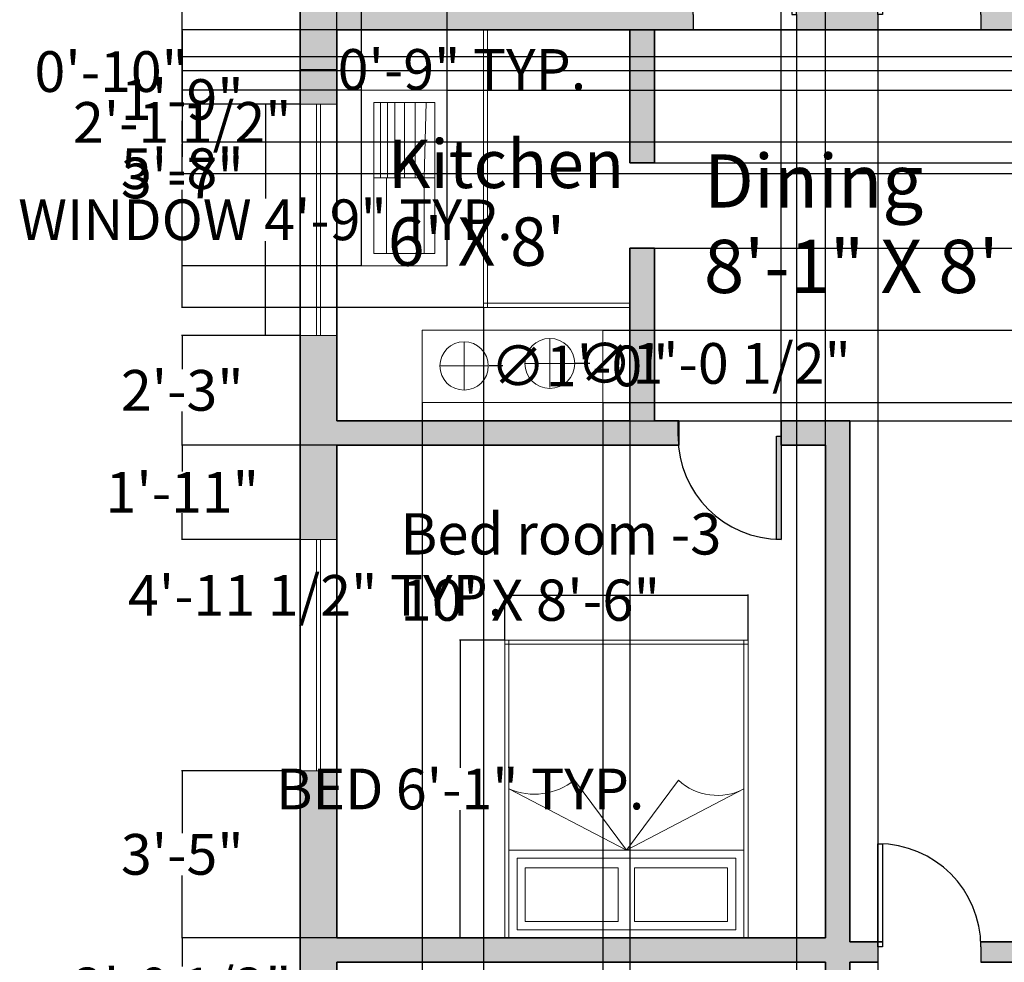
# Model space of a CAD drawing. Units: inches. Extents: x 46 to 946, y 121 to 740.
# Tile 2 of 4: x 46 to 287, y 299 to 531. Entities that reach past the tile are written whole.
import ezdxf

# ---------------------------------------------------------------- set-up
doc = ezdxf.new("R2010")
doc.units = ezdxf.units.IN
doc.header["$MEASUREMENT"] = 0
for name, color, linetype, lineweight in [('A-ANNO-DIMS', 2, 'Continuous', 18), ('A-AREA-IDEN', 7, 'Continuous', 25), ('A-DOOR', 3, 'Continuous', 25), ('A-EQPM', 9, 'Continuous', 18), ('A-FLOR-CASE', 8, 'Continuous', 18), ('A-FLOR-FIXT', 9, 'Continuous', 18), ('A-FURN', 8, 'Continuous', 18), ('A-GLAZ', 4, 'Continuous', 18), ('A-WALL', 7, 'Continuous', 35), ('A-WALL-PATT', 8, 'Continuous', 13)]:
    doc.layers.add(name, color=color, linetype=linetype, lineweight=lineweight)
doc.styles.get("Standard").update_dxf_attribs({"font": 'arial.ttf'})
doc.dimstyles.get("Standard").update_dxf_attribs({"dimtxt": 10, "dimasz": 0.18, "dimexe": 0.18, "dimexo": 0.0625, "dimgap": 0.09, "dimtad": 0, "dimtih": 1, "dimtoh": 1, "dimdec": 0, "dimzin": 0, "dimdsep": 46, "dimlunit": 3, "dimtxsty": 'Standard', "dimcen": 0.09, "dimadec": 0, "dimazin": 0, "dimtfac": 1, "dimtdec": 0, "dimtofl": 0, "dimtmove": 0, "dimatfit": 3, "dimfxl": 1, "dimtolj": 1, "dimtzin": 0, "dimarcsym": 0})

# ---------------------------------------------------------------- blocks, each defined once
blk = doc.blocks.new('*U3')
for p, q in [((0, 0), (0, -6)), ((40, 0), (40, -6))]:
    blk.add_line(p, q)
blk.add_lwpolyline([(0, 0), (0, 40), (1.75, 40), (1.75, 0)], close=True)
blk.add_arc((0, 0), 40, 0, 90)
blk = doc.blocks.new('WIN-56_82IN')
for p, q in [((9, 56.82), (0, 56.82)), ((0, 0), (0, 56.82)), ((4, 56.82), (4, 0)), ((5, 56.82), (5, 0)), ((9, 56.82), (9, 0)), ((9, 0), (0, 0))]:
    blk.add_line(p, q)
blk = doc.blocks.new('BED-DOUBLE')
for p, q in [((0, 73.15), (0, 0)), ((1, 73.15), (1, 0)), ((58.72, 0), (58.72, 73.15)), ((59.72, 0), (59.72, 73.15)), ((29.86, 51.59), (1, 36.57)), ((29.86, 51.59), (17.08, 34.42)), ((29.86, 51.59), (58.72, 36.57)), ((29.86, 51.59), (42.63, 34.42)), ((0, 1), (59.72, 1)), ((0, 0), (59.72, 0))]:
    blk.add_line(p, q)
for points in [[(1, 73.15), (58.72, 73.15), (58.72, 51.59), (1, 51.59)], [(3, 71.15), (56.72, 71.15), (56.72, 53.59), (3, 53.59)], [(5, 69.15), (27.85, 69.15), (27.85, 55.92), (5, 55.92)], [(54.72, 69.15), (31.87, 69.15), (31.87, 55.92), (54.72, 55.92)]]:
    blk.add_lwpolyline(points, close=True)
for centre, radius, start, end in [((7.51, 24.06), 14.1, 47.2425, 117.4957), ((52.47, 22.1), 15.76, 66.6553, 128.6065)]:
    blk.add_arc(centre, radius, start, end)
blk = doc.blocks.new('*D18')
at = {"layer": 'A-ANNO-DIMS', "color": 0, "lineweight": -2, "transparency": 16777216}
for p, q in [((114.41, 510.24), (105.77, 510.24)), ((105.95, 510.06), (105.95, 487.09)), ((105.95, 453.6), (105.95, 476.56)), ((114.41, 453.42), (105.77, 453.42))]:
    blk.add_line(p, q, dxfattribs=at)
at = {"layer": 'A-ANNO-DIMS', "color": 0, "transparency": 16777216}
for points in [[(105.92, 510.06), (105.98, 510.06), (105.95, 510.24)], [(105.92, 453.6), (105.98, 453.6), (105.95, 453.42)]]:
    blk.add_solid(points, dxfattribs=at)
at = {"layer": 'Defpoints', "color": 0, "transparency": 16777216}
for p in [(105.95, 510.24), (114.48, 510.24), (114.48, 453.42)]:
    blk.add_point(p, dxfattribs=at)
at = {"layer": 'A-ANNO-DIMS', "color": 0, "transparency": 16777216, "insert": (105.95, 481.83), "char_height": 10, "attachment_point": 5}
blk.add_mtext('\\A1;WINDOW 4\'-9" TYP.', dxfattribs=at)
blk = doc.blocks.new('*D19')
at = {"layer": 'A-ANNO-DIMS', "color": 0, "lineweight": -2, "transparency": 16777216}
for p, q in [((114.48, 510.3), (114.48, 518.94)), ((114.66, 518.76), (123.3, 518.76)), ((123.48, 510.3), (123.48, 518.94)), ((123.48, 518.76), (123.66, 518.76))]:
    blk.add_line(p, q, dxfattribs=at)
at = {"layer": 'A-ANNO-DIMS', "color": 0, "transparency": 16777216}
for points in [[(114.66, 518.79), (114.66, 518.73), (114.48, 518.76)], [(123.3, 518.79), (123.3, 518.73), (123.48, 518.76)]]:
    blk.add_solid(points, dxfattribs=at)
at = {"layer": 'Defpoints', "color": 0, "transparency": 16777216}
for p in [(123.48, 518.76), (114.48, 510.24), (123.48, 510.24)]:
    blk.add_point(p, dxfattribs=at)
at = {"layer": 'A-ANNO-DIMS', "color": 0, "transparency": 16777216, "insert": (154.22, 518.76), "char_height": 10, "attachment_point": 5}
blk.add_mtext('\\A1;0\'-9" TYP.', dxfattribs=at)
blk = doc.blocks.new('*D22')
at = {"layer": 'A-ANNO-DIMS', "color": 0, "lineweight": -2, "transparency": 16777216}
for p, q in [((164.7, 378.61), (153.61, 378.61)), ((153.79, 378.43), (153.79, 347.23)), ((153.79, 305.64), (153.79, 336.84)), ((164.7, 305.46), (153.61, 305.46))]:
    blk.add_line(p, q, dxfattribs=at)
at = {"layer": 'A-ANNO-DIMS', "color": 0, "transparency": 16777216}
for points in [[(153.76, 378.43), (153.82, 378.43), (153.79, 378.61)], [(153.76, 305.64), (153.82, 305.64), (153.79, 305.46)]]:
    blk.add_solid(points, dxfattribs=at)
at = {"layer": 'Defpoints', "color": 0, "transparency": 16777216}
for p in [(164.76, 378.61), (153.79, 305.46), (164.76, 305.46)]:
    blk.add_point(p, dxfattribs=at)
at = {"layer": 'A-ANNO-DIMS', "color": 0, "transparency": 16777216, "insert": (153.79, 342.03), "char_height": 10, "attachment_point": 5}
blk.add_mtext('\\A1;BED 6\'-1" TYP.', dxfattribs=at)
blk = doc.blocks.new('*D23')
at = {"layer": 'A-ANNO-DIMS', "color": 0, "lineweight": -2, "transparency": 16777216}
for p, q in [((164.76, 389.58), (164.58, 389.58)), ((164.76, 378.67), (164.76, 389.76)), ((224.3, 389.58), (164.94, 389.58)), ((224.48, 378.67), (224.48, 389.76))]:
    blk.add_line(p, q, dxfattribs=at)
at = {"layer": 'A-ANNO-DIMS', "color": 0, "transparency": 16777216}
for points in [[(164.94, 389.61), (164.94, 389.55), (164.76, 389.58)], [(224.3, 389.61), (224.3, 389.55), (224.48, 389.58)]]:
    blk.add_solid(points, dxfattribs=at)
at = {"layer": 'Defpoints', "color": 0, "transparency": 16777216}
for p in [(164.76, 389.58), (164.76, 378.61), (224.48, 378.61)]:
    blk.add_point(p, dxfattribs=at)
at = {"layer": 'A-ANNO-DIMS', "color": 0, "transparency": 16777216, "insert": (118.28, 389.58), "char_height": 10, "attachment_point": 5}
blk.add_mtext('\\A1;4\'-11 1/2" TYP.', dxfattribs=at)
blk = doc.blocks.new('*D32')
at = {"layer": 'A-ANNO-DIMS', "color": 0, "lineweight": -2, "transparency": 16777216}
for p, q in [((123.41, 305.46), (85.35, 305.46)), ((85.53, 305.28), (85.53, 298.41)), ((85.53, 281.01), (85.53, 287.89)), ((114.41, 280.83), (85.35, 280.83))]:
    blk.add_line(p, q, dxfattribs=at)
at = {"layer": 'A-ANNO-DIMS', "color": 0, "transparency": 16777216}
for points in [[(85.5, 305.28), (85.56, 305.28), (85.53, 305.46)], [(85.5, 281.01), (85.56, 281.01), (85.53, 280.83)]]:
    blk.add_solid(points, dxfattribs=at)
at = {"layer": 'Defpoints', "color": 0, "transparency": 16777216}
for p in [(85.53, 305.46), (123.48, 305.46), (114.48, 280.83)]:
    blk.add_point(p, dxfattribs=at)
at = {"layer": 'A-ANNO-DIMS', "color": 0, "transparency": 16777216, "insert": (85.53, 293.15), "char_height": 10, "attachment_point": 5}
blk.add_mtext('\\A1;2\'-0 1/2"', dxfattribs=at)
blk = doc.blocks.new('*D33')
at = {"layer": 'A-ANNO-DIMS', "color": 0, "lineweight": -2, "transparency": 16777216}
for p, q in [((114.41, 346.49), (85.35, 346.49)), ((85.53, 346.31), (85.53, 331.17)), ((85.53, 305.64), (85.53, 320.78)), ((123.41, 305.46), (85.35, 305.46))]:
    blk.add_line(p, q, dxfattribs=at)
at = {"layer": 'A-ANNO-DIMS', "color": 0, "transparency": 16777216}
for points in [[(85.5, 346.31), (85.56, 346.31), (85.53, 346.49)], [(85.5, 305.64), (85.56, 305.64), (85.53, 305.46)]]:
    blk.add_solid(points, dxfattribs=at)
at = {"layer": 'Defpoints', "color": 0, "transparency": 16777216}
for p in [(85.53, 346.49), (114.48, 346.49), (123.48, 305.46)]:
    blk.add_point(p, dxfattribs=at)
at = {"layer": 'A-ANNO-DIMS', "color": 0, "transparency": 16777216, "insert": (85.53, 325.98), "char_height": 10, "attachment_point": 5}
blk.add_mtext('\\A1;3\'-5"', dxfattribs=at)
blk = doc.blocks.new('*D34')
at = {"layer": 'A-ANNO-DIMS', "color": 0, "lineweight": -2, "transparency": 16777216}
for p, q in [((123.41, 426.46), (85.35, 426.46)), ((85.53, 426.28), (85.53, 420)), ((85.53, 403.49), (85.53, 409.78)), ((114.41, 403.31), (85.35, 403.31))]:
    blk.add_line(p, q, dxfattribs=at)
at = {"layer": 'A-ANNO-DIMS', "color": 0, "transparency": 16777216}
for points in [[(85.5, 426.28), (85.56, 426.28), (85.53, 426.46)], [(85.5, 403.49), (85.56, 403.49), (85.53, 403.31)]]:
    blk.add_solid(points, dxfattribs=at)
at = {"layer": 'Defpoints', "color": 0, "transparency": 16777216}
for p in [(85.53, 426.46), (123.48, 426.46), (114.48, 403.31)]:
    blk.add_point(p, dxfattribs=at)
at = {"layer": 'A-ANNO-DIMS', "color": 0, "transparency": 16777216, "insert": (85.53, 414.89), "char_height": 10, "attachment_point": 5}
blk.add_mtext('\\A1;1\'-11"', dxfattribs=at)
blk = doc.blocks.new('*D35')
at = {"layer": 'A-ANNO-DIMS', "color": 0, "lineweight": -2, "transparency": 16777216}
for p, q in [((114.41, 453.42), (85.35, 453.42)), ((85.53, 453.24), (85.53, 445.14)), ((85.53, 426.64), (85.53, 434.74)), ((123.41, 426.46), (85.35, 426.46))]:
    blk.add_line(p, q, dxfattribs=at)
at = {"layer": 'A-ANNO-DIMS', "color": 0, "transparency": 16777216}
for points in [[(85.5, 453.24), (85.56, 453.24), (85.53, 453.42)], [(85.5, 426.64), (85.56, 426.64), (85.53, 426.46)]]:
    blk.add_solid(points, dxfattribs=at)
at = {"layer": 'Defpoints', "color": 0, "transparency": 16777216}
for p in [(85.53, 453.42), (114.48, 453.42), (123.48, 426.46)]:
    blk.add_point(p, dxfattribs=at)
at = {"layer": 'A-ANNO-DIMS', "color": 0, "transparency": 16777216, "insert": (85.53, 439.94), "char_height": 10, "attachment_point": 5}
blk.add_mtext('\\A1;2\'-3"', dxfattribs=at)
blk = doc.blocks.new('*D36')
at = {"layer": 'A-ANNO-DIMS', "color": 0, "lineweight": -2, "transparency": 16777216}
for p, q in [((114.41, 573.18), (85.35, 573.18)), ((85.53, 573), (85.53, 546.91)), ((85.53, 510.42), (85.53, 536.51)), ((114.41, 510.24), (85.35, 510.24))]:
    blk.add_line(p, q, dxfattribs=at)
at = {"layer": 'A-ANNO-DIMS', "color": 0, "transparency": 16777216}
for points in [[(85.5, 573), (85.56, 573), (85.53, 573.18)], [(85.5, 510.42), (85.56, 510.42), (85.53, 510.24)]]:
    blk.add_solid(points, dxfattribs=at)
at = {"layer": 'Defpoints', "color": 0, "transparency": 16777216}
for p in [(85.53, 573.18), (114.48, 573.18), (114.48, 510.24)]:
    blk.add_point(p, dxfattribs=at)
at = {"layer": 'A-ANNO-DIMS', "color": 0, "transparency": 16777216, "insert": (85.53, 541.71), "char_height": 10, "attachment_point": 5}
blk.add_mtext('\\A1;5\'-3"', dxfattribs=at)
blk = doc.blocks.new('*D45')
at = {"layer": 'A-ANNO-DIMS', "color": 0, "lineweight": -2, "transparency": 16777216}
for p, q in [((129.58, 470.61), (129.58, 722.59)), ((129.76, 722.41), (150.42, 722.41)), ((150.6, 470.61), (150.6, 722.59)), ((150.6, 722.41), (150.78, 722.41))]:
    blk.add_line(p, q, dxfattribs=at)
at = {"layer": 'A-ANNO-DIMS', "color": 0, "transparency": 16777216}
for points in [[(129.76, 722.44), (129.76, 722.38), (129.58, 722.41)], [(150.42, 722.44), (150.42, 722.38), (150.6, 722.41)]]:
    blk.add_solid(points, dxfattribs=at)
at = {"layer": 'Defpoints', "color": 0, "transparency": 16777216}
for p in [(150.6, 722.41), (129.58, 470.54), (150.6, 470.54)]:
    blk.add_point(p, dxfattribs=at)
at = {"layer": 'A-ANNO-DIMS', "color": 0, "transparency": 16777216, "insert": (163.69, 722.41), "char_height": 10, "attachment_point": 5}
blk.add_mtext('\\A1;1\'-9"', dxfattribs=at)
blk = doc.blocks.new('*D46')
at = {"layer": 'A-ANNO-DIMS', "color": 0, "lineweight": -2, "transparency": 16777216}
for p, q in [((129.52, 513.68), (85.35, 513.68)), ((85.53, 513.5), (85.53, 497.31)), ((85.53, 470.72), (85.53, 486.91)), ((129.52, 470.54), (85.35, 470.54))]:
    blk.add_line(p, q, dxfattribs=at)
at = {"layer": 'A-ANNO-DIMS', "color": 0, "transparency": 16777216}
for points in [[(85.5, 513.5), (85.56, 513.5), (85.53, 513.68)], [(85.5, 470.72), (85.56, 470.72), (85.53, 470.54)]]:
    blk.add_solid(points, dxfattribs=at)
at = {"layer": 'Defpoints', "color": 0, "transparency": 16777216}
for p in [(85.53, 513.68), (129.58, 513.68), (129.58, 470.54)]:
    blk.add_point(p, dxfattribs=at)
at = {"layer": 'A-ANNO-DIMS', "color": 0, "transparency": 16777216, "insert": (85.53, 492.11), "char_height": 10, "attachment_point": 5}
blk.add_mtext('\\A1;3\'-7"', dxfattribs=at)
blk = doc.blocks.new('*D47')
at = {"layer": 'A-ANNO-DIMS', "color": 0, "lineweight": -2, "transparency": 16777216}
for p, q in [((144.44, 436.91), (144.44, 135.33)), ((188.83, 436.91), (188.83, 135.33)), ((144.62, 135.51), (188.65, 135.51)), ((188.83, 135.51), (189.01, 135.51))]:
    blk.add_line(p, q, dxfattribs=at)
at = {"layer": 'A-ANNO-DIMS', "color": 0, "transparency": 16777216}
for points in [[(144.62, 135.54), (144.62, 135.48), (144.44, 135.51)], [(188.65, 135.54), (188.65, 135.48), (188.83, 135.51)]]:
    blk.add_solid(points, dxfattribs=at)
at = {"layer": 'Defpoints', "color": 0, "transparency": 16777216}
for p in [(144.44, 436.97), (188.83, 436.97), (188.83, 135.51)]:
    blk.add_point(p, dxfattribs=at)
at = {"layer": 'A-ANNO-DIMS', "color": 0, "transparency": 16777216, "insert": (214.03, 135.51), "char_height": 10, "attachment_point": 5}
blk.add_mtext('\\A1;3\'-8 1/2"', dxfattribs=at)
blk = doc.blocks.new('*D48')
at = {"layer": 'A-ANNO-DIMS', "color": 0, "lineweight": -2, "transparency": 16777216}
for p, q in [((188.89, 454.75), (482.61, 454.75)), ((482.43, 454.57), (482.43, 451.05)), ((482.43, 437.15), (482.43, 440.66)), ((188.89, 436.97), (482.61, 436.97))]:
    blk.add_line(p, q, dxfattribs=at)
at = {"layer": 'A-ANNO-DIMS', "color": 0, "transparency": 16777216}
for points in [[(482.4, 454.57), (482.46, 454.57), (482.43, 454.75)], [(482.4, 437.15), (482.46, 437.15), (482.43, 436.97)]]:
    blk.add_solid(points, dxfattribs=at)
at = {"layer": 'Defpoints', "color": 0, "transparency": 16777216}
for p in [(188.83, 454.75), (482.43, 454.75), (188.83, 436.97)]:
    blk.add_point(p, dxfattribs=at)
at = {"layer": 'A-ANNO-DIMS', "color": 0, "transparency": 16777216, "insert": (482.43, 445.86), "char_height": 10, "attachment_point": 5}
blk.add_mtext('\\A1;1\'-6"', dxfattribs=at)
blk = doc.blocks.new('*D49')
at = {"layer": 'A-ANNO-DIMS', "color": 0, "lineweight": -2, "transparency": 16777216}
for p, q in [((159.48, 460.26), (159.48, 135.33)), ((195.48, 460.26), (195.48, 135.33)), ((159.66, 135.51), (164.1, 135.51)), ((195.3, 135.51), (190.85, 135.51))]:
    blk.add_line(p, q, dxfattribs=at)
at = {"layer": 'A-ANNO-DIMS', "color": 0, "transparency": 16777216}
for points in [[(159.66, 135.54), (159.66, 135.48), (159.48, 135.51)], [(195.3, 135.54), (195.3, 135.48), (195.48, 135.51)]]:
    blk.add_solid(points, dxfattribs=at)
at = {"layer": 'Defpoints', "color": 0, "transparency": 16777216}
for p in [(159.48, 460.32), (195.48, 460.32), (195.48, 135.51)]:
    blk.add_point(p, dxfattribs=at)
at = {"layer": 'A-ANNO-DIMS', "color": 0, "transparency": 16777216, "insert": (177.48, 135.51), "char_height": 10, "attachment_point": 5}
blk.add_mtext('\\A1;3\'-0"', dxfattribs=at)
blk = doc.blocks.new('*D50')
at = {"layer": 'A-ANNO-DIMS', "color": 0, "lineweight": -2, "transparency": 16777216}
for p, q in [((195.54, 495.84), (482.61, 495.84)), ((482.43, 495.66), (482.43, 490.57)), ((482.43, 475.08), (482.43, 480.18)), ((195.54, 474.9), (482.61, 474.9))]:
    blk.add_line(p, q, dxfattribs=at)
at = {"layer": 'A-ANNO-DIMS', "color": 0, "transparency": 16777216}
for points in [[(482.4, 495.66), (482.46, 495.66), (482.43, 495.84)], [(482.4, 475.08), (482.46, 475.08), (482.43, 474.9)]]:
    blk.add_solid(points, dxfattribs=at)
at = {"layer": 'Defpoints', "color": 0, "transparency": 16777216}
for p in [(195.48, 495.84), (482.43, 495.84), (195.48, 474.9)]:
    blk.add_point(p, dxfattribs=at)
at = {"layer": 'A-ANNO-DIMS', "color": 0, "transparency": 16777216, "insert": (482.43, 485.37), "char_height": 10, "attachment_point": 5}
blk.add_mtext('\\A1;1\'-9"', dxfattribs=at)
blk = doc.blocks.new('*D60')
at = {"layer": 'A-ANNO-DIMS', "color": 0, "lineweight": -2, "transparency": 16777216}
for p, q in [((385.41, 521.87), (85.35, 521.87)), ((85.53, 521.69), (85.53, 516.57)), ((85.53, 501.05), (85.53, 506.18)), ((385.41, 500.87), (85.35, 500.87))]:
    blk.add_line(p, q, dxfattribs=at)
at = {"layer": 'A-ANNO-DIMS', "color": 0, "transparency": 16777216}
for points in [[(85.5, 521.69), (85.56, 521.69), (85.53, 521.87)], [(85.5, 501.05), (85.56, 501.05), (85.53, 500.87)]]:
    blk.add_solid(points, dxfattribs=at)
at = {"layer": 'Defpoints', "color": 0, "transparency": 16777216}
for p in [(85.53, 521.87), (385.48, 521.87), (385.48, 500.87)]:
    blk.add_point(p, dxfattribs=at)
at = {"layer": 'A-ANNO-DIMS', "color": 0, "transparency": 16777216, "insert": (85.53, 511.37), "char_height": 10, "attachment_point": 5}
blk.add_mtext('\\A1;1\'-9"', dxfattribs=at)
blk = doc.blocks.new('*D61')
at = {"layer": 'A-ANNO-DIMS', "color": 0, "lineweight": -2, "transparency": 16777216}
for p, q in [((304.41, 528.46), (85.35, 528.46)), ((85.53, 528.28), (85.53, 518.59)), ((298.41, 518.41), (85.35, 518.41)), ((85.53, 518.23), (85.35, 518.23)), ((85.53, 518.41), (85.53, 518.23))]:
    blk.add_line(p, q, dxfattribs=at)
at = {"layer": 'A-ANNO-DIMS', "color": 0, "transparency": 16777216}
for points in [[(85.5, 528.28), (85.56, 528.28), (85.53, 528.46)], [(85.5, 518.59), (85.56, 518.59), (85.53, 518.41)]]:
    blk.add_solid(points, dxfattribs=at)
at = {"layer": 'Defpoints', "color": 0, "transparency": 16777216}
for p in [(304.48, 528.46), (85.53, 518.41), (298.48, 518.41)]:
    blk.add_point(p, dxfattribs=at)
at = {"layer": 'A-ANNO-DIMS', "color": 0, "transparency": 16777216, "insert": (68.08, 518.23), "char_height": 10, "attachment_point": 5}
blk.add_mtext('\\A1;0\'-10"', dxfattribs=at)
blk = doc.blocks.new('*D62')
at = {"layer": 'A-ANNO-DIMS', "color": 0, "lineweight": -2, "transparency": 16777216}
for p, q in [((298.41, 518.41), (85.35, 518.41)), ((85.53, 518.23), (85.53, 511.01)), ((85.53, 493.27), (85.53, 500.49)), ((298.41, 493.09), (85.35, 493.09))]:
    blk.add_line(p, q, dxfattribs=at)
at = {"layer": 'A-ANNO-DIMS', "color": 0, "transparency": 16777216}
for points in [[(85.5, 518.23), (85.56, 518.23), (85.53, 518.41)], [(85.5, 493.27), (85.56, 493.27), (85.53, 493.09)]]:
    blk.add_solid(points, dxfattribs=at)
at = {"layer": 'Defpoints', "color": 0, "transparency": 16777216}
for p in [(298.48, 518.41), (85.53, 493.09), (298.48, 493.09)]:
    blk.add_point(p, dxfattribs=at)
at = {"layer": 'A-ANNO-DIMS', "color": 0, "transparency": 16777216, "insert": (85.53, 505.75), "char_height": 10, "attachment_point": 5}
blk.add_mtext('\\A1;2\'-1 1/2"', dxfattribs=at)
blk = doc.blocks.new('*D63')
at = {"layer": 'A-ANNO-DIMS', "color": 0, "lineweight": -2, "transparency": 16777216}
for p, q in [((195.54, 528.46), (482.61, 528.46)), ((482.43, 528.28), (482.43, 517.41)), ((482.43, 496.02), (482.43, 506.89)), ((195.54, 495.84), (482.61, 495.84))]:
    blk.add_line(p, q, dxfattribs=at)
at = {"layer": 'A-ANNO-DIMS', "color": 0, "transparency": 16777216}
for points in [[(482.4, 528.28), (482.46, 528.28), (482.43, 528.46)], [(482.4, 496.02), (482.46, 496.02), (482.43, 495.84)]]:
    blk.add_solid(points, dxfattribs=at)
at = {"layer": 'Defpoints', "color": 0, "transparency": 16777216}
for p in [(195.48, 528.46), (195.48, 495.84), (482.43, 495.84)]:
    blk.add_point(p, dxfattribs=at)
at = {"layer": 'A-ANNO-DIMS', "color": 0, "transparency": 16777216, "insert": (482.43, 512.15), "char_height": 10, "attachment_point": 5}
blk.add_mtext('\\A1;2\'-8 1/2"', dxfattribs=at)
blk = doc.blocks.new('*D64')
at = {"layer": 'A-ANNO-DIMS', "color": 0, "lineweight": -2, "transparency": 16777216}
for p, q in [((188.83, 436.91), (188.83, 135.33)), ((195.48, 432.4), (195.48, 135.33)), ((188.83, 135.51), (188.65, 135.51)), ((195.3, 135.51), (189.01, 135.51))]:
    blk.add_line(p, q, dxfattribs=at)
at = {"layer": 'A-ANNO-DIMS', "color": 0, "transparency": 16777216}
for points in [[(189.01, 135.54), (189.01, 135.48), (188.83, 135.51)], [(195.3, 135.54), (195.3, 135.48), (195.48, 135.51)]]:
    blk.add_solid(points, dxfattribs=at)
at = {"layer": 'Defpoints', "color": 0, "transparency": 16777216}
for p in [(188.83, 436.97), (195.48, 432.46), (188.83, 135.51)]:
    blk.add_point(p, dxfattribs=at)
at = {"layer": 'A-ANNO-DIMS', "color": 0, "transparency": 16777216, "insert": (163.61, 135.51), "char_height": 10, "attachment_point": 5}
blk.add_mtext('\\A1;0\'-6 1/2"', dxfattribs=at)
blk = doc.blocks.new('*D65')
at = {"layer": 'A-ANNO-DIMS', "color": 0, "lineweight": -2, "transparency": 16777216}
for p, q in [((232.61, 426.52), (232.61, 722.59)), ((232.79, 722.41), (243.3, 722.41)), ((243.48, 426.52), (243.48, 722.59)), ((243.48, 722.41), (243.66, 722.41))]:
    blk.add_line(p, q, dxfattribs=at)
at = {"layer": 'A-ANNO-DIMS', "color": 0, "transparency": 16777216}
for points in [[(232.79, 722.44), (232.79, 722.38), (232.61, 722.41)], [(243.3, 722.44), (243.3, 722.38), (243.48, 722.41)]]:
    blk.add_solid(points, dxfattribs=at)
at = {"layer": 'Defpoints', "color": 0, "transparency": 16777216}
for p in [(243.48, 722.41), (232.61, 426.46), (243.48, 426.46)]:
    blk.add_point(p, dxfattribs=at)
at = {"layer": 'A-ANNO-DIMS', "color": 0, "transparency": 16777216, "insert": (260.92, 722.41), "char_height": 10, "attachment_point": 5}
blk.add_mtext('\\A1;0\'-11"', dxfattribs=at)
blk = doc.blocks.new('*D66')
at = {"layer": 'A-ANNO-DIMS', "color": 0, "lineweight": -2, "transparency": 16777216}
for p, q in [((123.48, 528.52), (123.48, 722.59)), ((123.66, 722.41), (129.4, 722.41)), ((129.58, 513.74), (129.58, 722.59)), ((129.58, 722.41), (129.76, 722.41))]:
    blk.add_line(p, q, dxfattribs=at)
at = {"layer": 'A-ANNO-DIMS', "color": 0, "transparency": 16777216}
for points in [[(123.66, 722.44), (123.66, 722.38), (123.48, 722.41)], [(129.4, 722.44), (129.4, 722.38), (129.58, 722.41)]]:
    blk.add_solid(points, dxfattribs=at)
at = {"layer": 'Defpoints', "color": 0, "transparency": 16777216}
for p in [(129.58, 722.41), (123.48, 528.46), (129.58, 513.68)]:
    blk.add_point(p, dxfattribs=at)
at = {"layer": 'A-ANNO-DIMS', "color": 0, "transparency": 16777216, "insert": (143.14, 722.41), "char_height": 10, "attachment_point": 5}
blk.add_mtext('\\A1;0\'-6"', dxfattribs=at)
blk = doc.blocks.new('*D67')
at = {"layer": 'A-ANNO-DIMS', "color": 0, "lineweight": -2, "transparency": 16777216}
for p, q in [((159.54, 528.46), (482.61, 528.46)), ((482.43, 528.28), (482.43, 526.27)), ((482.43, 513.86), (482.43, 515.87)), ((150.66, 513.68), (482.61, 513.68))]:
    blk.add_line(p, q, dxfattribs=at)
at = {"layer": 'A-ANNO-DIMS', "color": 0, "transparency": 16777216}
for points in [[(482.4, 528.28), (482.46, 528.28), (482.43, 528.46)], [(482.4, 513.86), (482.46, 513.86), (482.43, 513.68)]]:
    blk.add_solid(points, dxfattribs=at)
at = {"layer": 'Defpoints', "color": 0, "transparency": 16777216}
for p in [(159.48, 528.46), (482.43, 528.46), (150.6, 513.68)]:
    blk.add_point(p, dxfattribs=at)
at = {"layer": 'A-ANNO-DIMS', "color": 0, "transparency": 16777216, "insert": (482.43, 521.07), "char_height": 10, "attachment_point": 5}
blk.add_mtext('\\A1;1\'-3"', dxfattribs=at)
blk = doc.blocks.new('*D68')
at = {"layer": 'A-ANNO-DIMS', "color": 0, "lineweight": -2, "transparency": 16777216}
for p, q in [((159.41, 528.46), (85.35, 528.46)), ((85.53, 528.28), (85.53, 499.59)), ((85.53, 460.5), (85.53, 489.2)), ((159.41, 460.32), (85.35, 460.32))]:
    blk.add_line(p, q, dxfattribs=at)
at = {"layer": 'A-ANNO-DIMS', "color": 0, "transparency": 16777216}
for points in [[(85.5, 528.28), (85.56, 528.28), (85.53, 528.46)], [(85.5, 460.5), (85.56, 460.5), (85.53, 460.32)]]:
    blk.add_solid(points, dxfattribs=at)
at = {"layer": 'Defpoints', "color": 0, "transparency": 16777216}
for p in [(159.48, 528.46), (85.53, 460.32), (159.48, 460.32)]:
    blk.add_point(p, dxfattribs=at)
at = {"layer": 'A-ANNO-DIMS', "color": 0, "transparency": 16777216, "insert": (85.53, 494.39), "char_height": 10, "attachment_point": 5}
blk.add_mtext('\\A1;5\'-8"', dxfattribs=at)
blk = doc.blocks.new('*D69')
at = {"layer": 'A-ANNO-DIMS', "color": 0, "lineweight": -2, "transparency": 16777216}
for p, q in [((188.89, 436.97), (482.61, 436.97)), ((482.43, 436.79), (482.43, 432.64)), ((195.54, 432.46), (482.61, 432.46)), ((482.43, 432.28), (482.25, 432.28)), ((482.43, 432.46), (482.43, 432.28))]:
    blk.add_line(p, q, dxfattribs=at)
at = {"layer": 'A-ANNO-DIMS', "color": 0, "transparency": 16777216}
for points in [[(482.4, 436.79), (482.46, 436.79), (482.43, 436.97)], [(482.4, 432.64), (482.46, 432.64), (482.43, 432.46)]]:
    blk.add_solid(points, dxfattribs=at)
at = {"layer": 'Defpoints', "color": 0, "transparency": 16777216}
for p in [(188.83, 436.97), (195.48, 432.46), (482.43, 432.46)]:
    blk.add_point(p, dxfattribs=at)
at = {"layer": 'A-ANNO-DIMS', "color": 0, "transparency": 16777216, "insert": (457.21, 432.28), "char_height": 10, "attachment_point": 5}
blk.add_mtext('\\A1;0\'-4 1/2"', dxfattribs=at)
blk = doc.blocks.new('*D70')
at = {"layer": 'A-ANNO-DIMS', "color": 0, "lineweight": -2, "transparency": 16777216}
for p, q in [((236.36, 528.4), (236.36, 135.33)), ((256.37, 528.4), (256.37, 135.33)), ((236.54, 135.51), (256.19, 135.51)), ((256.37, 135.51), (256.55, 135.51))]:
    blk.add_line(p, q, dxfattribs=at)
at = {"layer": 'A-ANNO-DIMS', "color": 0, "transparency": 16777216}
for points in [[(236.54, 135.54), (236.54, 135.48), (236.36, 135.51)], [(256.19, 135.54), (256.19, 135.48), (256.37, 135.51)]]:
    blk.add_solid(points, dxfattribs=at)
at = {"layer": 'Defpoints', "color": 0, "transparency": 16777216}
for p in [(236.36, 528.46), (256.37, 528.46), (256.37, 135.51)]:
    blk.add_point(p, dxfattribs=at)
at = {"layer": 'A-ANNO-DIMS', "color": 0, "transparency": 16777216, "insert": (269.46, 135.51), "char_height": 10, "attachment_point": 5}
blk.add_mtext('\\A1;1\'-8"', dxfattribs=at)
blk = doc.blocks.new('*D71')
at = {"layer": 'A-ANNO-DIMS', "color": 0, "lineweight": -2, "transparency": 16777216}
for p, q in [((175.72, 446.56), (175.9, 446.56)), ((175.81, 446.47), (175.81, 446.65)), ((185.61, 446.56), (182.12, 446.56))]:
    blk.add_line(p, q, dxfattribs=at)
at = {"layer": 'A-ANNO-DIMS', "color": 0, "transparency": 16777216}
blk.add_solid([(182.12, 446.59), (182.12, 446.53), (181.94, 446.56)], dxfattribs=at)
at = {"layer": 'Defpoints', "color": 0, "transparency": 16777216}
for p in [(169.68, 446.56), (181.94, 446.56)]:
    blk.add_point(p, dxfattribs=at)
at = {"layer": 'A-ANNO-DIMS', "color": 0, "transparency": 16777216, "insert": (216.09, 446.56), "char_height": 10, "attachment_point": 5}
blk.add_mtext('\\A1;∅1\'-0 1/2"', dxfattribs=at)
blk = doc.blocks.new('*D72')
at = {"layer": 'A-ANNO-DIMS', "color": 0, "lineweight": -2, "transparency": 16777216}
for p, q in [((154.66, 445.94), (154.84, 445.94)), ((154.75, 445.85), (154.75, 446.03)), ((164.27, 445.94), (160.88, 445.94))]:
    blk.add_line(p, q, dxfattribs=at)
at = {"layer": 'A-ANNO-DIMS', "color": 0, "transparency": 16777216}
blk.add_solid([(160.88, 445.97), (160.88, 445.91), (160.7, 445.94)], dxfattribs=at)
at = {"layer": 'Defpoints', "color": 0, "transparency": 16777216}
for p in [(148.8, 445.94), (160.7, 445.94)]:
    blk.add_point(p, dxfattribs=at)
at = {"layer": 'A-ANNO-DIMS', "color": 0, "transparency": 16777216, "insert": (183.09, 445.94), "char_height": 10, "attachment_point": 5}
blk.add_mtext('\\A1;∅1\'-0"', dxfattribs=at)

msp = doc.modelspace()

# ---------------------------------------------------------------- hatches: boundary and pattern name
at = {"layer": 'A-WALL-PATT'}
h = msp.add_hatch(color=256, dxfattribs=at)
h.dxf.hatch_style = 1
h.paths.add_polyline_path([(256.37, 197.46), (249.48, 197.46), (249.48, 258.28), (245.68, 258.28, -0.021769), (243.48, 258.37), (243.48, 197.46), (221.61, 197.46), (221.61, 188.46), (243.48, 188.46), (256.37, 188.46), (256.37, 192.26)])
h.paths.add_polyline_path([(164.78, 197.46), (123.48, 197.46), (123.48, 224.01), (114.48, 224.01), (114.48, 188.46), (164.78, 188.46)])
h.paths.add_polyline_path([(402.48, 216.63), (393.48, 216.63), (393.48, 197.46), (327.48, 197.46), (281.15, 197.46, -0.051771), (281.69, 192.26), (281.69, 188.46), (402.48, 188.46)])
h.paths.add_polyline_path([(123.48, 346.49), (114.48, 346.49), (114.48, 280.83), (123.48, 280.83), (123.48, 299.46), (243.48, 299.46), (243.48, 283.6), (245.68, 283.6), (249.48, 283.6), (249.48, 299.46), (256.37, 299.46), (256.37, 303.26), (256.37, 304.46), (249.48, 304.46), (249.48, 432.46), (243.48, 432.46), (232.61, 432.46), (232.61, 426.46), (243.48, 426.46), (243.48, 305.46), (123.48, 305.46)])
h.paths.add_polyline_path([(231.5, 428.66), (232.61, 428.66), (232.61, 403.34), (231.5, 403.34), (231.5, 403.37, -0.376395), (207.38, 426.46), (123.48, 426.46), (123.48, 403.31), (114.48, 403.31), (114.48, 453.42), (123.48, 453.42), (123.48, 432.46), (195.48, 432.46), (195.48, 474.9), (201.48, 474.9), (201.48, 432.46), (207.29, 432.46), (207.29, 428.66, 0.401453), (231.5, 403.37)])
h.paths.add_polyline_path([(211.14, 534.46), (123.48, 534.46), (123.48, 573.18), (114.48, 573.18), (114.48, 510.24), (123.48, 510.24), (123.48, 528.46), (195.48, 528.46), (195.48, 495.84), (201.48, 495.84), (201.48, 528.46), (211.04, 528.46), (211.04, 532.26, -0.021769)])
h.paths.add_polyline_path([(123.48, 684.46), (243.48, 684.46), (243.48, 534.46), (236.36, 534.46), (236.36, 532.26), (236.36, 528.46), (256.37, 528.46), (256.37, 532.26), (256.37, 534.46), (249.48, 534.46), (249.48, 684.46), (393.48, 684.46), (393.48, 647.42), (402.48, 647.42), (402.48, 693.46), (114.48, 693.46), (114.48, 630), (123.48, 630)])
h.paths.add_polyline_path([(402.48, 590.59), (393.48, 590.59), (393.48, 534.46), (281.59, 534.46, -0.021769), (281.69, 532.26), (281.69, 528.46), (298.48, 528.46), (298.48, 518.41), (302.28, 518.41), (304.48, 518.41), (304.48, 528.46), (393.48, 528.46), (393.48, 518.87), (402.48, 518.87)])
h.paths.add_polyline_path([(402.48, 500.87), (393.48, 500.87), (393.48, 482.46), (304.48, 482.46), (304.48, 493.19, -0.021769), (302.28, 493.09), (298.48, 493.09), (298.48, 482.46), (298.48, 476.46), (304.48, 476.46), (393.48, 476.46), (393.48, 455.17), (402.48, 455.17)])
h.paths.add_polyline_path([(402.48, 419.17), (393.48, 419.17), (393.48, 356.8), (402.48, 356.8)])
h.paths.add_polyline_path([(358.48, 304.46), (281.66, 304.46, -0.01187), (281.69, 303.26), (281.69, 299.46), (358.48, 299.46)])

# ---------------------------------------------------------------- linework, layer by layer
at = {"layer": 'A-EQPM'}
for p, q in [((175.81, 452.51), (175.81, 440.61)), ((154.75, 451.89), (154.75, 439.99)), ((160.7, 445.94), (148.8, 445.94)), ((154.75, 439.99), (154.75, 445.94)), ((154.75, 445.94), (160.7, 445.94)), ((181.76, 446.56), (169.86, 446.56)), ((175.81, 440.61), (175.81, 446.56))]:
    msp.add_line(p, q, dxfattribs=at)
msp.add_lwpolyline([(188.83, 436.97), (144.44, 436.97), (144.44, 454.75), (188.83, 454.75)], close=True, dxfattribs=at)
for centre, radius in [((175.81, 446.56), 6.13), ((154.75, 445.94), 5.95)]:
    msp.add_circle(centre, radius, dxfattribs=at)
at = {"layer": 'A-FLOR-CASE'}
for p, q in [((159.48, 528.46), (159.48, 460.32)), ((160.48, 528.46), (160.48, 460.32)), ((159.48, 461.32), (195.48, 461.32)), ((159.48, 460.32), (195.48, 460.32))]:
    msp.add_line(p, q, dxfattribs=at)
at = {"layer": 'A-FLOR-FIXT'}
for p, q in [((134.2, 492.11), (134.2, 510.68)), ((134.2, 510.68), (135.97, 510.68)), ((135.97, 510.68), (135.97, 492.11)), ((137.74, 492.11), (137.74, 510.68)), ((137.74, 510.68), (140.09, 510.68)), ((140.09, 510.68), (140.09, 492.11)), ((142.7, 492.11), (142.7, 510.68)), ((142.7, 510.68), (145.45, 510.68)), ((145.45, 510.68), (144.97, 492.11)), ((132.58, 492.11), (147.6, 492.11)), ((144.97, 492.11), (135.68, 492.11)), ((135.68, 492.11), (135.68, 473.54)), ((135.97, 492.11), (137.74, 492.11)), ((140.09, 492.11), (142.7, 492.11)), ((144.97, 473.54), (144.97, 492.11)), ((147.6, 492.11), (147.6, 473.54)), ((147.6, 473.54), (144.97, 473.54))]:
    msp.add_line(p, q, dxfattribs=at)
for points in [[(129.58, 513.68), (150.6, 513.68), (150.6, 470.54), (129.58, 470.54)], [(132.58, 510.68), (147.6, 510.68), (147.6, 473.54), (132.58, 473.54)]]:
    msp.add_lwpolyline(points, close=True, dxfattribs=at)
at = {"layer": 'A-WALL'}
for p, q in [((114.48, 693.46), (114.48, 188.46)), ((123.48, 528.46), (195.48, 528.46)), ((123.48, 528.46), (123.48, 432.46)), ((195.48, 528.46), (195.48, 495.84)), ((201.48, 528.46), (201.48, 495.84)), ((201.48, 528.46), (211.04, 528.46)), ((236.36, 528.46), (256.37, 528.46)), ((281.69, 528.46), (298.48, 528.46)), ((195.48, 495.84), (201.48, 495.84)), ((201.48, 474.9), (195.48, 474.9)), ((195.48, 474.9), (195.48, 432.46)), ((201.48, 474.9), (201.48, 432.46)), ((123.48, 432.46), (195.48, 432.46)), ((201.48, 432.46), (207.48, 432.46)), ((207.48, 432.46), (207.29, 432.46)), ((207.48, 432.46), (207.48, 426.46)), ((243.48, 432.46), (232.61, 432.46)), ((232.61, 432.46), (232.61, 426.46)), ((243.48, 432.46), (249.48, 432.46)), ((249.48, 432.46), (249.48, 304.46)), ((123.48, 426.46), (195.48, 426.46)), ((207.48, 426.46), (123.48, 426.46)), ((123.48, 426.46), (123.48, 305.46)), ((207.48, 426.46), (207.48, 426.46)), ((232.61, 426.46), (243.48, 426.46)), ((243.48, 426.46), (243.48, 305.46)), ((243.48, 305.46), (123.48, 305.46)), ((257.48, 304.46), (249.48, 304.46)), ((393.48, 304.46), (281.66, 304.46)), ((123.48, 299.46), (123.48, 197.46)), ((123.48, 299.46), (243.48, 299.46)), ((243.48, 299.46), (243.48, 282.49)), ((243.48, 299.46), (243.48, 282.49)), ((249.48, 299.46), (249.48, 283.6)), ((249.48, 299.46), (256.37, 299.46)), ((281.69, 299.46), (393.48, 299.46))]:
    msp.add_line(p, q, dxfattribs=at)

# ---------------------------------------------------------------- block references
at = {"layer": 'A-DOOR', "yscale": 0.6330408260540115, "zscale": 0.6330408260540115}
for p, xscale in [((236.36, 532.26), -0.6330408260540115), ((256.37, 532.26), 0.6330408260540115), ((256.37, 303.26), 0.6330408260540115)]:
    msp.add_blockref('*U3', p, dxfattribs=dict(at, xscale=xscale))
at = {"layer": 'A-DOOR', "xscale": 0.6330408260540115, "yscale": 0.6330408260540115, "zscale": 0.6330408260540115, "rotation": 179.9999999999998}
msp.add_blockref('*U3', (232.61, 428.66), dxfattribs=at)
at = {"layer": 'A-FURN', "rotation": 180}
msp.add_blockref('BED-DOUBLE', (224.48, 378.61), dxfattribs=at)
at = {"layer": 'A-GLAZ'}
for p in [(114.48, 453.42), (114.48, 346.49)]:
    msp.add_blockref('WIN-56_82IN', p, dxfattribs=at)

# ---------------------------------------------------------------- texts
at = {"layer": 'A-AREA-IDEN'}
for s, height, p in [('Kitchen', 11.882, (136.02, 489.63)), ('Dining', 13.067, (213.65, 484.84)), ("6' X 8'", 11.882, (136.02, 470.54)), ('8\'-1" X 8\'', 13.067, (213.65, 463.85)), ('Bed room -3', 10.1255, (139.11, 399.62)), ('10\' X 8\'-6"', 10.1255, (139.11, 383.35))]:
    msp.add_text(s, height=height, dxfattribs=at).set_placement(p)

# ---------------------------------------------------------------- dimensions: what is measured, and where the dimension line sits
at = {"layer": 'A-ANNO-DIMS'}
for base, p1, p2, picture, middle in [((129.58, 722.41), (123.48, 528.46), (129.58, 513.68), '*D66', (143.14, 722.41)), ((150.6, 722.41), (129.58, 470.54), (150.6, 470.54), '*D45', (163.69, 722.41)), ((243.48, 722.41), (232.61, 426.46), (243.48, 426.46), '*D65', (260.92, 722.41)), ((256.37, 135.51), (236.36, 528.46), (256.37, 528.46), '*D70', (269.46, 135.51)), ((195.48, 135.51), (159.48, 460.32), (195.48, 460.32), '*D49', (177.48, 135.51)), ((188.8251, 135.5113), (195.4768, 432.4613), (188.8251, 436.9697), '*D64', (163.6131, 135.5113)), ((188.83, 135.51), (144.44, 436.97), (188.83, 436.97), '*D47', (214.03, 135.51))]:
    dim = msp.add_linear_dim(base=base, p1=p1, p2=p2, dimstyle='Standard', override={"dimdec": 1, "dimlfac": 1, "dimrnd": 0, "dimzin": 1, "dimdsep": 46, "dimlunit": 4, "dimfrac": 2}, dxfattribs=at)
    dim.commit()
    dim.dimension.update_dxf_attribs({"geometry": picture, "text_midpoint": middle})
for base, p1, p2, picture, middle in [((85.53, 573.18), (114.48, 510.24), (114.48, 573.18), '*D36', (85.53, 541.71)), ((85.5268, 518.4133), (304.4768, 528.4613), (298.4768, 518.4133), '*D61', (68.0808, 518.2333)), ((85.53, 460.32), (159.48, 528.46), (159.48, 460.32), '*D68', (85.53, 494.39)), ((482.43, 528.46), (150.6, 513.68), (159.48, 528.46), '*D67', (482.43, 521.07)), ((482.43, 495.84), (195.48, 528.46), (195.48, 495.84), '*D63', (482.43, 512.15)), ((85.53, 493.09), (298.48, 518.41), (298.48, 493.09), '*D62', (85.53, 505.75)), ((85.53, 521.87), (385.48, 500.87), (385.48, 521.87), '*D60', (85.53, 511.37)), ((85.53, 513.68), (129.58, 470.54), (129.58, 513.68), '*D46', (85.53, 492.11)), ((482.43, 495.84), (195.48, 474.9), (195.48, 495.84), '*D50', (482.43, 485.37)), ((482.43, 454.75), (188.83, 436.97), (188.83, 454.75), '*D48', (482.43, 445.86)), ((85.53, 453.42), (123.48, 426.46), (114.48, 453.42), '*D35', (85.53, 439.94)), ((482.43, 432.46), (188.83, 436.97), (195.48, 432.46), '*D69', (457.21, 432.28)), ((85.5268, 426.4613), (114.4768, 403.3108), (123.4768, 426.4613), '*D34', (85.5268, 414.8861)), ((85.53, 346.49), (123.48, 305.46), (114.48, 346.49), '*D33', (85.53, 325.98)), ((85.53, 305.46), (114.48, 280.83), (123.48, 305.46), '*D32', (85.53, 293.15))]:
    dim = msp.add_linear_dim(base=base, p1=p1, p2=p2, angle=90, dimstyle='Standard', override={"dimdec": 1, "dimlfac": 1, "dimrnd": 0, "dimzin": 1, "dimdsep": 46, "dimlunit": 4, "dimfrac": 2}, dxfattribs=at)
    dim.commit()
    dim.dimension.update_dxf_attribs({"geometry": picture, "text_midpoint": middle})
dim = msp.add_linear_dim(base=(123.48, 518.76), p1=(114.48, 510.24), p2=(123.48, 510.24), text='<> TYP.', dimstyle='Standard', override={"dimdec": 1, "dimlfac": 1, "dimrnd": 0, "dimzin": 1, "dimdsep": 46, "dimlunit": 4, "dimfrac": 2}, dxfattribs=at)
dim.commit()
dim.dimension.update_dxf_attribs({"geometry": '*D19', "text_midpoint": (154.22, 518.76)})
for base, p1, p2, angle, text, picture, middle in [((105.95, 510.24), (114.48, 453.42), (114.48, 510.24), 90, 'WINDOW <> TYP.', '*D18', (105.95, 481.83)), ((164.76, 389.58), (224.48, 378.61), (164.76, 378.61), 180, '<> TYP.', '*D23', (118.28, 389.58)), ((153.788, 305.4613), (164.7597, 378.6064), (164.7597, 305.4613), 270, 'BED <> TYP.', '*D22', (153.788, 342.0339))]:
    dim = msp.add_linear_dim(base=base, p1=p1, p2=p2, angle=angle, text=text, dimstyle='Standard', override={"dimdec": 1, "dimlfac": 1, "dimrnd": 0, "dimzin": 1, "dimdsep": 46, "dimlunit": 4, "dimfrac": 2}, dxfattribs=at)
    dim.commit()
    dim.dimension.update_dxf_attribs({"geometry": picture, "text_midpoint": middle})
for p1, p2, picture, middle in [((169.68, 446.56), (181.94, 446.56), '*D71', (185.61, 446.56)), ((148.8, 445.94), (160.7, 445.94), '*D72', (164.27, 445.94))]:
    dim = msp.add_diameter_dim_2p(p1=p1, p2=p2, dimstyle='Standard', override={"dimdec": 1, "dimlfac": 1, "dimrnd": 0, "dimzin": 1, "dimdsep": 46, "dimlunit": 4, "dimfrac": 2}, dxfattribs=at)
    dim.commit()
    dim.dimension.update_dxf_attribs({"geometry": picture, "text_midpoint": middle, "dimtype": 163})

doc.saveas('drawing.dxf')
